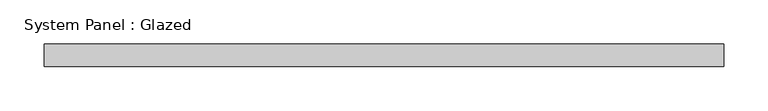
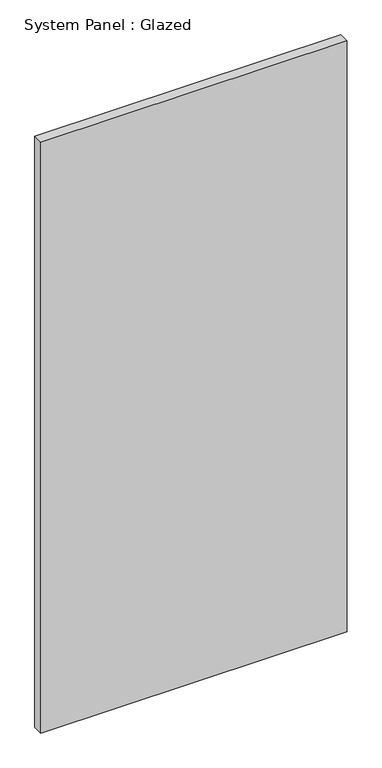
"""IFC4 building model written with IfcOpenShell, lengths in millimetres: plate geometry, System Panel : Glazed."""

from ifc_helpers import new_model, si_unit, origin, origin_with_axes, place, context, project, spatial, polyline, outline, extrude, source, transform, mapped, element, save


def system_panel_glazed_7ff316d0(model_context):
    return source(origin(), model_context, "Body", "SweptSolid", [
        extrude(outline(polyline([(384.175, 19.05), (-384.175, 19.05), (-384.175, 44.45), (384.175, 44.45), (384.175, 19.05)])), origin_with_axes(), (0.0, 0.0, 1.0), 1566.6943888),
    ])


if __name__ == "__main__":
    model = new_model("IFC4")
    model_context = context("Model", 3, world=origin())
    ifc_project = project(units=[si_unit("LENGTHUNIT", "METRE", prefix="MILLI")], contexts=[model_context])
    site = spatial("IfcSite", under=ifc_project)
    building = spatial("IfcBuilding", under=site)
    placement = place(None, origin())
    system_panel_glazed_shape = system_panel_glazed_7ff316d0(model_context)
    element("IfcPlate", 1, ObjectType="System Panel : Glazed", at=placement, inside=building, context=model_context, shape_type="MappedRepresentation", body=[
        mapped(system_panel_glazed_shape, transform((0.0, 0.0, 0.0), x_axis=(1.0, 0.0, 0.0), y_axis=(0.0, 1.0, 0.0), z_axis=(0.0, 0.0, 1.0))),
    ])
    save(model, "model.ifc")

# Revit data of these elements
# Type "System Panel : Glazed"
#   Construction Type Id = "GSP4R"
#   Analytic Construction = "1/8 in Pilkington single glazing"
#   Visual Light Transmittance = 0.9
#   Solar Heat Gain Coefficient = 0.86
#   Heat Transfer Coefficient (U) = 1.18115 BTU/(h·ft²·°F)
#   Define Thermal Properties by = 1
# Element 1 (IfcPlate, "System Panel : Glazed")
#   Materials on its faces: "Glass"
# Materials
#   "Glass": class "Glass", colour RGB 0 128 192, transparency 0.75, Description = "Soda Lime Glass", Cost = 0
